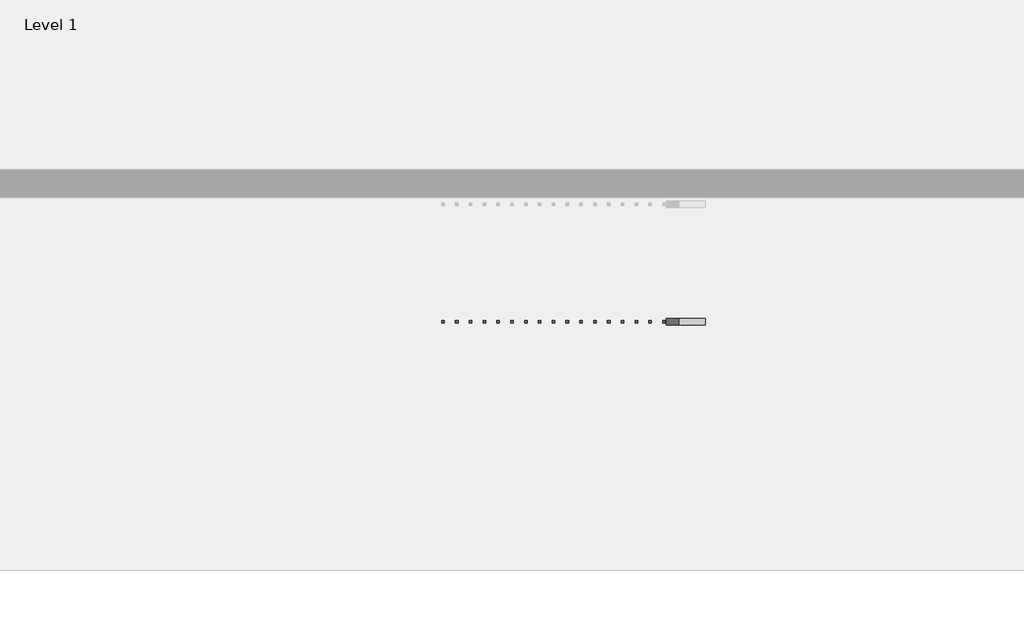
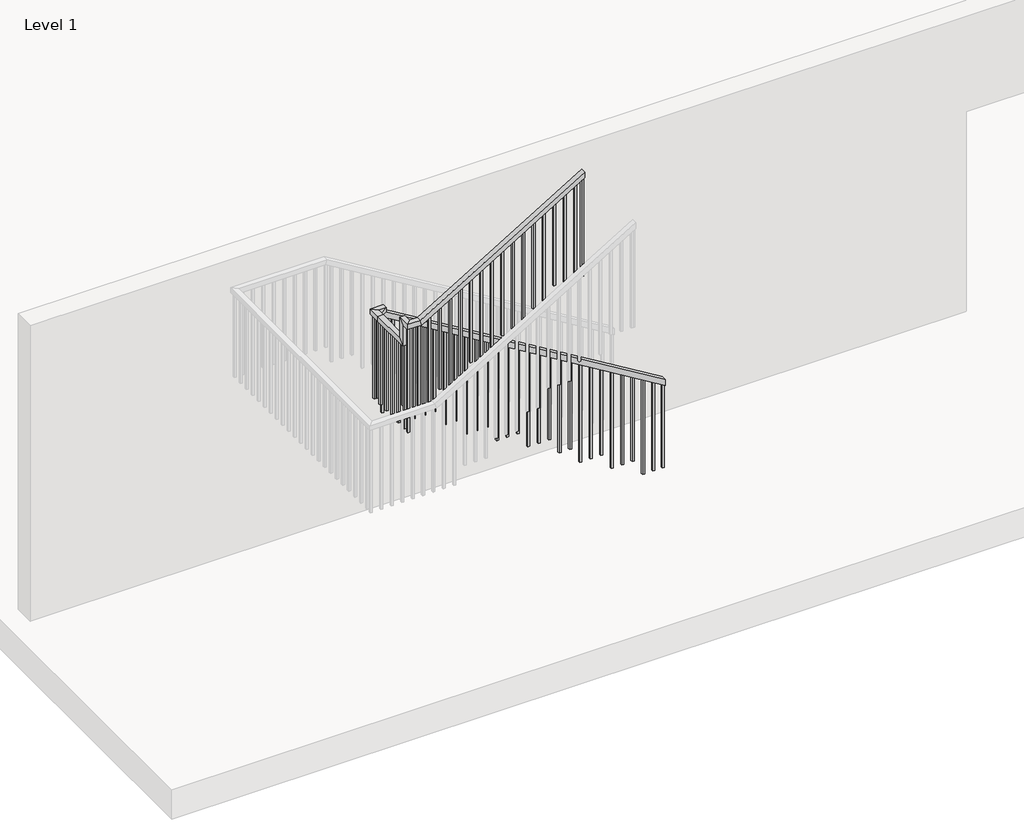
# One storey, part 2 of 2: 1 railing.
"""IFC4 building model written with IfcOpenShell, lengths in millimetres."""

from ifc_helpers import new_model, si_unit, frame, origin, place, context, project, spatial, polyline, outline, extrude, faceted_brep, element, save

model = new_model("IFC4")

# Units and contexts
model_context = context("Model", 3, world=origin())
ifc_project = project(units=[si_unit("LENGTHUNIT", "METRE", prefix="MILLI")], contexts=[model_context])

# Site, building, storey
site = spatial("IfcSite", under=ifc_project)
building = spatial("IfcBuilding", under=site)
storey = spatial("IfcBuildingStorey", under=building, Name="Level 1", Elevation=0.0)

# Railing
placement = place(None, origin())
element("IfcRailing", 1, ObjectType="Handrail - Rectangular", at=placement, inside=storey, context=model_context, shape_type="SolidModel", body=[
    faceted_brep([(-5944.3382419, -6921.2242744, 1083.7333333), (-5944.3382419, -6921.2242744, 1024.3318731), (-5944.3382419, -6870.4242744, 1024.3318731), (-5944.3382419, -6870.4242744, 1083.7333333), (-8662.1382419, -6921.2242744, 2730.8848485), (-8712.9382419, -6921.2242744, 2702.271267), (-8712.9382419, -6870.4242744, 2702.271267), (-8662.1382419, -6870.4242744, 2730.8848485), (-8738.3382419, -6997.4242744, 2726.2666667), (-8738.3382419, -6997.4242744, 2777.0666667), (-8738.3382419, -7366.3243151, 2777.0666667), (-8738.3382419, -7417.1243151, 2726.2666667), (-8789.1382419, -6997.4242744, 2726.2666667), (-8789.1382419, -7417.1243151, 2726.2666667), (-8789.1382419, -6997.4242744, 2777.0666667), (-8789.1382419, -7366.3243151, 2777.0666667), (-7061.9382419, -7442.5243151, 3962.4), (-7061.9382419, -7493.3243151, 3962.4), (-7061.9382419, -7493.3243151, 3902.9985397), (-7061.9382419, -7442.5243151, 3902.9985397), (-8647.9458325, -7442.5243151, 2941.7818182), (-8662.1382419, -7442.5243151, 2992.5818182), (-8647.9458325, -7493.3243151, 2941.7818182), (-8662.1382419, -7493.3243151, 2992.5818182), (-8662.1382419, -6921.2242744, 2777.0666667), (-8712.9382419, -6921.2242744, 2726.2666667), (-8712.9382419, -6870.4242744, 2726.2666667), (-8662.1382419, -6870.4242744, 2777.0666667), (-8738.3382419, -6921.2242744, 2777.0666667), (-8738.3382419, -6921.2242744, 2726.2666667), (-8789.1382419, -6870.4242744, 2726.2666667), (-8789.1382419, -6870.4242744, 2777.0666667), (-8738.3382419, -7366.3243151, 2992.5818182), (-8738.3382419, -7417.1243151, 2941.7818182), (-8789.1382419, -7417.1243151, 2941.7818182), (-8789.1382419, -7366.3243151, 2992.5818182), (-8738.3382419, -7442.5243151, 2992.5818182), (-8738.3382419, -7442.5243151, 2941.7818182), (-8789.1382419, -7493.3243151, 2941.7818182), (-8789.1382419, -7493.3243151, 2992.5818182)], [[[0, 1, 2, 3]], [[1, 0, 4, 5]], [[2, 1, 5, 6]], [[3, 2, 6, 7]], [[0, 3, 7, 4]], [[8, 9, 10, 11]], [[12, 8, 11, 13]], [[14, 12, 13, 15]], [[9, 14, 15, 10]], [[16, 17, 18, 19]], [[20, 21, 16, 19]], [[22, 20, 19, 18]], [[23, 22, 18, 17]], [[21, 23, 17, 16]], [[5, 4, 24, 25]], [[6, 5, 25, 26]], [[7, 6, 26, 27]], [[4, 7, 27, 24]], [[25, 24, 28, 29]], [[26, 25, 29, 30]], [[27, 26, 30, 31]], [[24, 27, 31, 28]], [[29, 28, 9, 8]], [[30, 29, 8, 12]], [[31, 30, 12, 14]], [[28, 31, 14, 9]], [[11, 10, 32, 33]], [[13, 11, 33, 34]], [[15, 13, 34, 35]], [[10, 15, 35, 32]], [[33, 32, 36, 37]], [[34, 33, 37, 38]], [[35, 34, 38, 39]], [[32, 35, 39, 36]], [[37, 36, 21, 20]], [[38, 37, 20, 22]], [[39, 38, 22, 23]], [[36, 39, 23, 21]]]),
    extrude(outline(polyline([(3851.0439943, -7147.6632419), (2878.6666667, -7147.6632419), (2878.6666667, -7128.6132419), (3862.5894488, -7128.6132419), (3851.0439943, -7147.6632419)])), frame((0.0, -7477.4493151, 0.0), z_axis=(0.0, 1.0, 0.0), x_axis=(0.0, 0.0, 1.0)), (0.0, 0.0, 1.0), 19.05),
    extrude(outline(polyline([(3789.4682367, -7249.2632419), (2878.6666667, -7249.2632419), (2878.6666667, -7230.2132419), (3801.0136913, -7230.2132419), (3789.4682367, -7249.2632419)])), frame((0.0, -7477.4493151, 0.0), z_axis=(0.0, 1.0, 0.0), x_axis=(0.0, 0.0, 1.0)), (0.0, 0.0, 1.0), 19.05),
    extrude(outline(polyline([(3727.8924791, -7350.8632419), (2878.6666667, -7350.8632419), (2878.6666667, -7331.8132419), (3739.4379337, -7331.8132419), (3727.8924791, -7350.8632419)])), frame((0.0, -7477.4493151, 0.0), z_axis=(0.0, 1.0, 0.0), x_axis=(0.0, 0.0, 1.0)), (0.0, 0.0, 1.0), 19.05),
    extrude(outline(polyline([(3666.3167216, -7452.4632419), (2709.3333333, -7452.4632419), (2709.3333333, -7433.4132419), (3677.8621761, -7433.4132419), (3666.3167216, -7452.4632419)])), frame((0.0, -7477.4493151, 0.0), z_axis=(0.0, 1.0, 0.0), x_axis=(0.0, 0.0, 1.0)), (0.0, 0.0, 1.0), 19.05),
    extrude(outline(polyline([(3604.740964, -7554.0632419), (2709.3333333, -7554.0632419), (2709.3333333, -7535.0132419), (3616.2864185, -7535.0132419), (3604.740964, -7554.0632419)])), frame((0.0, -7477.4493151, 0.0), z_axis=(0.0, 1.0, 0.0), x_axis=(0.0, 0.0, 1.0)), (0.0, 0.0, 1.0), 19.05),
    extrude(outline(polyline([(3543.1652064, -7655.6632419), (2540.0, -7655.6632419), (2540.0, -7636.6132419), (3554.710661, -7636.6132419), (3543.1652064, -7655.6632419)])), frame((0.0, -7477.4493151, 0.0), z_axis=(0.0, 1.0, 0.0), x_axis=(0.0, 0.0, 1.0)), (0.0, 0.0, 1.0), 19.05),
    extrude(outline(polyline([(3481.5894488, -7757.2632419), (2540.0, -7757.2632419), (2540.0, -7738.2132419), (3493.1349034, -7738.2132419), (3481.5894488, -7757.2632419)])), frame((0.0, -7477.4493151, 0.0), z_axis=(0.0, 1.0, 0.0), x_axis=(0.0, 0.0, 1.0)), (0.0, 0.0, 1.0), 19.05),
    extrude(outline(polyline([(3420.0136913, -7858.8632419), (2540.0, -7858.8632419), (2540.0, -7839.8132419), (3431.5591458, -7839.8132419), (3420.0136913, -7858.8632419)])), frame((0.0, -7477.4493151, 0.0), z_axis=(0.0, 1.0, 0.0), x_axis=(0.0, 0.0, 1.0)), (0.0, 0.0, 1.0), 19.05),
    extrude(outline(polyline([(3358.4379337, -7960.4632419), (2370.6666667, -7960.4632419), (2370.6666667, -7941.4132419), (3369.9833882, -7941.4132419), (3358.4379337, -7960.4632419)])), frame((0.0, -7477.4493151, 0.0), z_axis=(0.0, 1.0, 0.0), x_axis=(0.0, 0.0, 1.0)), (0.0, 0.0, 1.0), 19.05),
    extrude(outline(polyline([(3296.8621761, -8062.0632419), (2370.6666667, -8062.0632419), (2370.6666667, -8043.0132419), (3308.4076307, -8043.0132419), (3296.8621761, -8062.0632419)])), frame((0.0, -7477.4493151, 0.0), z_axis=(0.0, 1.0, 0.0), x_axis=(0.0, 0.0, 1.0)), (0.0, 0.0, 1.0), 19.05),
    extrude(outline(polyline([(3235.2864185, -8163.6632419), (2370.6666667, -8163.6632419), (2370.6666667, -8144.6132419), (3246.8318731, -8144.6132419), (3235.2864185, -8163.6632419)])), frame((0.0, -7477.4493151, 0.0), z_axis=(0.0, 1.0, 0.0), x_axis=(0.0, 0.0, 1.0)), (0.0, 0.0, 1.0), 19.05),
    extrude(outline(polyline([(3173.710661, -8265.2632419), (2201.3333333, -8265.2632419), (2201.3333333, -8246.2132419), (3185.2561155, -8246.2132419), (3173.710661, -8265.2632419)])), frame((0.0, -7477.4493151, 0.0), z_axis=(0.0, 1.0, 0.0), x_axis=(0.0, 0.0, 1.0)), (0.0, 0.0, 1.0), 19.05),
    extrude(outline(polyline([(3112.1349034, -8366.8632419), (2201.3333333, -8366.8632419), (2201.3333333, -8347.8132419), (3123.6803579, -8347.8132419), (3112.1349034, -8366.8632419)])), frame((0.0, -7477.4493151, 0.0), z_axis=(0.0, 1.0, 0.0), x_axis=(0.0, 0.0, 1.0)), (0.0, 0.0, 1.0), 19.05),
    extrude(outline(polyline([(3050.5591458, -8468.4632419), (2201.3333333, -8468.4632419), (2201.3333333, -8449.4132419), (3062.1046004, -8449.4132419), (3050.5591458, -8468.4632419)])), frame((0.0, -7477.4493151, 0.0), z_axis=(0.0, 1.0, 0.0), x_axis=(0.0, 0.0, 1.0)), (0.0, 0.0, 1.0), 19.05),
    extrude(outline(polyline([(2988.9833882, -8570.0632419), (2032.0, -8570.0632419), (2032.0, -8551.0132419), (3000.5288428, -8551.0132419), (2988.9833882, -8570.0632419)])), frame((0.0, -7477.4493151, 0.0), z_axis=(0.0, 1.0, 0.0), x_axis=(0.0, 0.0, 1.0)), (0.0, 0.0, 1.0), 19.05),
    extrude(outline(polyline([(-8671.6632419, -7458.3993151), (-8652.6132419, -7458.3993151), (-8652.6132419, -7477.4493151), (-8671.6632419, -7477.4493151), (-8671.6632419, -7458.3993151)])), frame((0.0, 0.0, 2032.0), z_axis=(0.0, 0.0, 1.0), x_axis=(1.0, 0.0, 0.0)), (0.0, 0.0, 1.0), 909.7818182),
    extrude(outline(polyline([(-8754.2132419, -7394.2992744), (-8754.2132419, -7413.3492744), (-8773.2632419, -7413.3492744), (-8773.2632419, -7394.2992744), (-8754.2132419, -7394.2992744)])), frame((0.0, 0.0, 1862.6666667), z_axis=(0.0, 0.0, 1.0), x_axis=(1.0, 0.0, 0.0)), (0.0, 0.0, 1.0), 863.6),
    extrude(outline(polyline([(-8754.2132419, -7292.6992744), (-8754.2132419, -7311.7492744), (-8773.2632419, -7311.7492744), (-8773.2632419, -7292.6992744), (-8754.2132419, -7292.6992744)])), frame((0.0, 0.0, 1862.6666667), z_axis=(0.0, 0.0, 1.0), x_axis=(1.0, 0.0, 0.0)), (0.0, 0.0, 1.0), 863.6),
    extrude(outline(polyline([(-8754.2132419, -7191.0992744), (-8754.2132419, -7210.1492744), (-8773.2632419, -7210.1492744), (-8773.2632419, -7191.0992744), (-8754.2132419, -7191.0992744)])), frame((0.0, 0.0, 1862.6666667), z_axis=(0.0, 0.0, 1.0), x_axis=(1.0, 0.0, 0.0)), (0.0, 0.0, 1.0), 863.6),
    extrude(outline(polyline([(-8754.2132419, -7089.4992744), (-8754.2132419, -7108.5492744), (-8773.2632419, -7108.5492744), (-8773.2632419, -7089.4992744), (-8754.2132419, -7089.4992744)])), frame((0.0, 0.0, 1862.6666667), z_axis=(0.0, 0.0, 1.0), x_axis=(1.0, 0.0, 0.0)), (0.0, 0.0, 1.0), 863.6),
    extrude(outline(polyline([(-8754.2132419, -6987.8992744), (-8754.2132419, -7006.9492744), (-8773.2632419, -7006.9492744), (-8773.2632419, -6987.8992744), (-8754.2132419, -6987.8992744)])), frame((0.0, 0.0, 1862.6666667), z_axis=(0.0, 0.0, 1.0), x_axis=(1.0, 0.0, 0.0)), (0.0, 0.0, 1.0), 863.6),
    extrude(outline(polyline([(2692.6500549, -8697.0632419), (1693.3333333, -8697.0632419), (1693.3333333, -8678.0132419), (2681.1046004, -8678.0132419), (2692.6500549, -8697.0632419)])), frame((0.0, -6905.3492744, 0.0), z_axis=(0.0, 1.0, 0.0), x_axis=(0.0, 0.0, 1.0)), (0.0, 0.0, 1.0), 19.05),
    extrude(outline(polyline([(2631.0742973, -8595.4632419), (1693.3333333, -8595.4632419), (1693.3333333, -8576.4132419), (2619.5288428, -8576.4132419), (2631.0742973, -8595.4632419)])), frame((0.0, -6905.3492744, 0.0), z_axis=(0.0, 1.0, 0.0), x_axis=(0.0, 0.0, 1.0)), (0.0, 0.0, 1.0), 19.05),
    extrude(outline(polyline([(2569.4985397, -8493.8632419), (1693.3333333, -8493.8632419), (1693.3333333, -8474.8132419), (2557.9530852, -8474.8132419), (2569.4985397, -8493.8632419)])), frame((0.0, -6905.3492744, 0.0), z_axis=(0.0, 1.0, 0.0), x_axis=(0.0, 0.0, 1.0)), (0.0, 0.0, 1.0), 19.05),
    extrude(outline(polyline([(2507.9227822, -8392.2632419), (1524.0, -8392.2632419), (1524.0, -8373.2132419), (2496.3773276, -8373.2132419), (2507.9227822, -8392.2632419)])), frame((0.0, -6905.3492744, 0.0), z_axis=(0.0, 1.0, 0.0), x_axis=(0.0, 0.0, 1.0)), (0.0, 0.0, 1.0), 19.05),
    extrude(outline(polyline([(2446.3470246, -8290.6632419), (1524.0, -8290.6632419), (1524.0, -8271.6132419), (2434.80157, -8271.6132419), (2446.3470246, -8290.6632419)])), frame((0.0, -6905.3492744, 0.0), z_axis=(0.0, 1.0, 0.0), x_axis=(0.0, 0.0, 1.0)), (0.0, 0.0, 1.0), 19.05),
    extrude(outline(polyline([(2384.771267, -8189.0632419), (1524.0, -8189.0632419), (1524.0, -8170.0132419), (2373.2258125, -8170.0132419), (2384.771267, -8189.0632419)])), frame((0.0, -6905.3492744, 0.0), z_axis=(0.0, 1.0, 0.0), x_axis=(0.0, 0.0, 1.0)), (0.0, 0.0, 1.0), 19.05),
    extrude(outline(polyline([(2323.1955094, -8087.4632419), (1354.6666667, -8087.4632419), (1354.6666667, -8068.4132419), (2311.6500549, -8068.4132419), (2323.1955094, -8087.4632419)])), frame((0.0, -6905.3492744, 0.0), z_axis=(0.0, 1.0, 0.0), x_axis=(0.0, 0.0, 1.0)), (0.0, 0.0, 1.0), 19.05),
    extrude(outline(polyline([(2261.6197519, -7985.8632419), (1354.6666667, -7985.8632419), (1354.6666667, -7966.8132419), (2250.0742973, -7966.8132419), (2261.6197519, -7985.8632419)])), frame((0.0, -6905.3492744, 0.0), z_axis=(0.0, 1.0, 0.0), x_axis=(0.0, 0.0, 1.0)), (0.0, 0.0, 1.0), 19.05),
    extrude(outline(polyline([(2200.0439943, -7884.2632419), (1185.3333333, -7884.2632419), (1185.3333333, -7865.2132419), (2188.4985397, -7865.2132419), (2200.0439943, -7884.2632419)])), frame((0.0, -6905.3492744, 0.0), z_axis=(0.0, 1.0, 0.0), x_axis=(0.0, 0.0, 1.0)), (0.0, 0.0, 1.0), 19.05),
    extrude(outline(polyline([(2138.4682367, -7782.6632419), (1185.3333333, -7782.6632419), (1185.3333333, -7763.6132419), (2126.9227822, -7763.6132419), (2138.4682367, -7782.6632419)])), frame((0.0, -6905.3492744, 0.0), z_axis=(0.0, 1.0, 0.0), x_axis=(0.0, 0.0, 1.0)), (0.0, 0.0, 1.0), 19.05),
    extrude(outline(polyline([(2076.8924791, -7681.0632419), (1185.3333333, -7681.0632419), (1185.3333333, -7662.0132419), (2065.3470246, -7662.0132419), (2076.8924791, -7681.0632419)])), frame((0.0, -6905.3492744, 0.0), z_axis=(0.0, 1.0, 0.0), x_axis=(0.0, 0.0, 1.0)), (0.0, 0.0, 1.0), 19.05),
    extrude(outline(polyline([(2015.3167216, -7579.4632419), (1016.0, -7579.4632419), (1016.0, -7560.4132419), (2003.771267, -7560.4132419), (2015.3167216, -7579.4632419)])), frame((0.0, -6905.3492744, 0.0), z_axis=(0.0, 1.0, 0.0), x_axis=(0.0, 0.0, 1.0)), (0.0, 0.0, 1.0), 19.05),
    extrude(outline(polyline([(1953.740964, -7477.8632419), (1016.0, -7477.8632419), (1016.0, -7458.8132419), (1942.1955094, -7458.8132419), (1953.740964, -7477.8632419)])), frame((0.0, -6905.3492744, 0.0), z_axis=(0.0, 1.0, 0.0), x_axis=(0.0, 0.0, 1.0)), (0.0, 0.0, 1.0), 19.05),
    extrude(outline(polyline([(1892.1652064, -7376.2632419), (1016.0, -7376.2632419), (1016.0, -7357.2132419), (1880.6197519, -7357.2132419), (1892.1652064, -7376.2632419)])), frame((0.0, -6905.3492744, 0.0), z_axis=(0.0, 1.0, 0.0), x_axis=(0.0, 0.0, 1.0)), (0.0, 0.0, 1.0), 19.05),
    extrude(outline(polyline([(1830.5894488, -7274.6632419), (846.6666667, -7274.6632419), (846.6666667, -7255.6132419), (1819.0439943, -7255.6132419), (1830.5894488, -7274.6632419)])), frame((0.0, -6905.3492744, 0.0), z_axis=(0.0, 1.0, 0.0), x_axis=(0.0, 0.0, 1.0)), (0.0, 0.0, 1.0), 19.05),
    extrude(outline(polyline([(1769.0136913, -7173.0632419), (846.6666667, -7173.0632419), (846.6666667, -7154.0132419), (1757.4682367, -7154.0132419), (1769.0136913, -7173.0632419)])), frame((0.0, -6905.3492744, 0.0), z_axis=(0.0, 1.0, 0.0), x_axis=(0.0, 0.0, 1.0)), (0.0, 0.0, 1.0), 19.05),
    extrude(outline(polyline([(1707.4379337, -7071.4632419), (846.6666667, -7071.4632419), (846.6666667, -7052.4132419), (1695.8924791, -7052.4132419), (1707.4379337, -7071.4632419)])), frame((0.0, -6905.3492744, 0.0), z_axis=(0.0, 1.0, 0.0), x_axis=(0.0, 0.0, 1.0)), (0.0, 0.0, 1.0), 19.05),
    extrude(outline(polyline([(1645.8621761, -6969.8632419), (677.3333333, -6969.8632419), (677.3333333, -6950.8132419), (1634.3167216, -6950.8132419), (1645.8621761, -6969.8632419)])), frame((0.0, -6905.3492744, 0.0), z_axis=(0.0, 1.0, 0.0), x_axis=(0.0, 0.0, 1.0)), (0.0, 0.0, 1.0), 19.05),
    extrude(outline(polyline([(1584.2864185, -6868.2632419), (677.3333333, -6868.2632419), (677.3333333, -6849.2132419), (1572.740964, -6849.2132419), (1584.2864185, -6868.2632419)])), frame((0.0, -6905.3492744, 0.0), z_axis=(0.0, 1.0, 0.0), x_axis=(0.0, 0.0, 1.0)), (0.0, 0.0, 1.0), 19.05),
    extrude(outline(polyline([(1522.710661, -6766.6632419), (508.0, -6766.6632419), (508.0, -6747.6132419), (1511.1652064, -6747.6132419), (1522.710661, -6766.6632419)])), frame((0.0, -6905.3492744, 0.0), z_axis=(0.0, 1.0, 0.0), x_axis=(0.0, 0.0, 1.0)), (0.0, 0.0, 1.0), 19.05),
    extrude(outline(polyline([(1461.1349034, -6665.0632419), (508.0, -6665.0632419), (508.0, -6646.0132419), (1449.5894488, -6646.0132419), (1461.1349034, -6665.0632419)])), frame((0.0, -6905.3492744, 0.0), z_axis=(0.0, 1.0, 0.0), x_axis=(0.0, 0.0, 1.0)), (0.0, 0.0, 1.0), 19.05),
    extrude(outline(polyline([(1399.5591458, -6563.4632419), (508.0, -6563.4632419), (508.0, -6544.4132419), (1388.0136913, -6544.4132419), (1399.5591458, -6563.4632419)])), frame((0.0, -6905.3492744, 0.0), z_axis=(0.0, 1.0, 0.0), x_axis=(0.0, 0.0, 1.0)), (0.0, 0.0, 1.0), 19.05),
    extrude(outline(polyline([(1337.9833882, -6461.8632419), (338.6666667, -6461.8632419), (338.6666667, -6442.8132419), (1326.4379337, -6442.8132419), (1337.9833882, -6461.8632419)])), frame((0.0, -6905.3492744, 0.0), z_axis=(0.0, 1.0, 0.0), x_axis=(0.0, 0.0, 1.0)), (0.0, 0.0, 1.0), 19.05),
    extrude(outline(polyline([(1276.4076307, -6360.2632419), (338.6666667, -6360.2632419), (338.6666667, -6341.2132419), (1264.8621761, -6341.2132419), (1276.4076307, -6360.2632419)])), frame((0.0, -6905.3492744, 0.0), z_axis=(0.0, 1.0, 0.0), x_axis=(0.0, 0.0, 1.0)), (0.0, 0.0, 1.0), 19.05),
    extrude(outline(polyline([(1214.8318731, -6258.6632419), (338.6666667, -6258.6632419), (338.6666667, -6239.6132419), (1203.2864185, -6239.6132419), (1214.8318731, -6258.6632419)])), frame((0.0, -6905.3492744, 0.0), z_axis=(0.0, 1.0, 0.0), x_axis=(0.0, 0.0, 1.0)), (0.0, 0.0, 1.0), 19.05),
    extrude(outline(polyline([(1153.2561155, -6157.0632419), (169.3333333, -6157.0632419), (169.3333333, -6138.0132419), (1141.710661, -6138.0132419), (1153.2561155, -6157.0632419)])), frame((0.0, -6905.3492744, 0.0), z_axis=(0.0, 1.0, 0.0), x_axis=(0.0, 0.0, 1.0)), (0.0, 0.0, 1.0), 19.05),
    extrude(outline(polyline([(1091.6803579, -6055.4632419), (169.3333333, -6055.4632419), (169.3333333, -6036.4132419), (1080.1349034, -6036.4132419), (1091.6803579, -6055.4632419)])), frame((0.0, -6905.3492744, 0.0), z_axis=(0.0, 1.0, 0.0), x_axis=(0.0, 0.0, 1.0)), (0.0, 0.0, 1.0), 19.05),
    extrude(outline(polyline([(-8773.2632419, -7458.3993151), (-8754.2132419, -7458.3993151), (-8754.2132419, -7477.4493151), (-8773.2632419, -7477.4493151), (-8773.2632419, -7458.3993151)])), frame((0.0, 0.0, 1862.6666667), z_axis=(0.0, 0.0, 1.0), x_axis=(1.0, 0.0, 0.0)), (0.0, 0.0, 1.0), 1079.1151515),
    extrude(outline(polyline([(-8754.2132419, -6905.3492744), (-8773.2632419, -6905.3492744), (-8773.2632419, -6886.2992744), (-8754.2132419, -6886.2992744), (-8754.2132419, -6905.3492744)])), frame((0.0, 0.0, 1862.6666667), z_axis=(0.0, 0.0, 1.0), x_axis=(1.0, 0.0, 0.0)), (0.0, 0.0, 1.0), 863.6),
    extrude(outline(polyline([(-8728.8132419, -6905.3492744), (-8747.8632419, -6905.3492744), (-8747.8632419, -6886.2992744), (-8728.8132419, -6886.2992744), (-8728.8132419, -6905.3492744)])), frame((0.0, 0.0, 1862.6666667), z_axis=(0.0, 0.0, 1.0), x_axis=(1.0, 0.0, 0.0)), (0.0, 0.0, 1.0), 863.6),
    extrude(outline(polyline([(3891.4530852, -7080.9882419), (2878.6666667, -7080.9882419), (2878.6666667, -7061.9382419), (3902.9985397, -7061.9382419), (3891.4530852, -7080.9882419)])), frame((0.0, -7477.4493151, 0.0), z_axis=(0.0, 1.0, 0.0), x_axis=(0.0, 0.0, 1.0)), (0.0, 0.0, 1.0), 19.05),
    extrude(outline(polyline([(1035.8773276, -5963.3882419), (169.3333333, -5963.3882419), (169.3333333, -5944.3382419), (1024.3318731, -5944.3382419), (1035.8773276, -5963.3882419)])), frame((0.0, -6905.3492744, 0.0), z_axis=(0.0, 1.0, 0.0), x_axis=(0.0, 0.0, 1.0)), (0.0, 0.0, 1.0), 19.05),
])

save(model, "model.ifc")

# Revit data of these elements
# Type "Handrail - Rectangular"
#   Assembly Code = "C2010400"
#   built-in parameter 1008612 = 0.0416667 (stored number, unit not read)
#   built-in parameter 1008611 = 0.0416667 (stored number, unit not read)
#   built-in parameter 1008609 = 0.333333 (stored number, unit not read)
#   built-in parameter 1008604 = 0.166667 (stored number, unit not read)
#   built-in parameter 1008603 = 0.166667 (stored number, unit not read)
#   Railing Height = 3' - 0"
#   built-in parameter 1008630 = 2
#   built-in parameter 1008610 = 2
#   built-in parameter 1008618 = Baluster - Square : 3/4"
# Element 1 (IfcRailing, "Handrail - Rectangular")
#   Phase Created = New Construction
